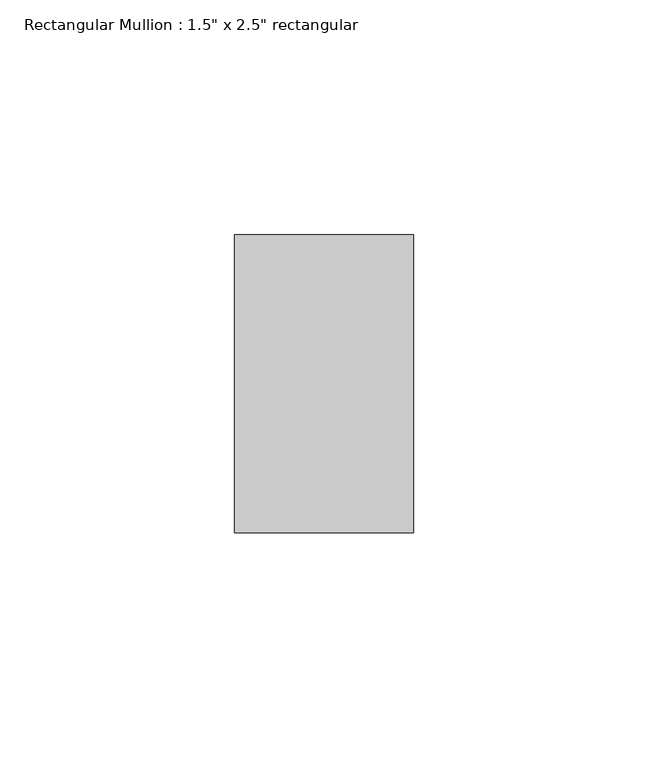
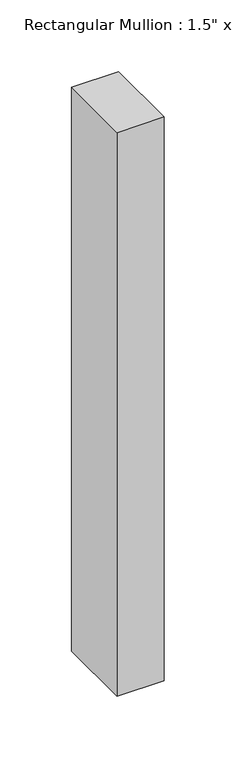
"""IFC4 building model written with IfcOpenShell, lengths in millimetres: member geometry."""

from ifc_helpers import new_model, si_unit, frame, origin, place, context, project, spatial, polyline, outline, extrude, source, transform, mapped, element, save


def member_6a2c51b8(model_context):
    return source(origin(), model_context, "Body", "SweptSolid", [
        extrude(outline(polyline([(19.05, 31.75), (19.05, -31.75), (-19.05, -31.75), (-19.05, 31.75), (19.05, 31.75)])), frame((0.0, 0.0, -480.1854569), z_axis=(0.0, 0.0, 1.0), x_axis=(1.0, 0.0, 0.0)), (0.0, 0.0, 1.0), 480.1854569),
    ])


if __name__ == "__main__":
    model = new_model("IFC4")
    model_context = context("Model", 3, world=origin())
    ifc_project = project(units=[si_unit("LENGTHUNIT", "METRE", prefix="MILLI")], contexts=[model_context])
    site = spatial("IfcSite", under=ifc_project)
    building = spatial("IfcBuilding", under=site)
    placement = place(None, origin())
    member_shape = member_6a2c51b8(model_context)
    element("IfcMember", 1, ObjectType="Rectangular Mullion : 1.5\" x 2.5\" rectangular", at=placement, inside=building, context=model_context, shape_type="MappedRepresentation", body=[
        mapped(member_shape, transform((0.0, 0.0, 0.0), x_axis=(1.0, 0.0, 0.0), y_axis=(0.0, 1.0, 0.0), z_axis=(0.0, 0.0, 1.0))),
    ])
    save(model, "model.ifc")

# Revit data of these elements
# Type "Rectangular Mullion : 1.5\" x 2.5\" rectangular"
#   built-in parameter 1007304 = 0.208333 (stored number, unit not read)
#   built-in parameter 1007301 = 0.0625 (stored number, unit not read)
#   built-in parameter 1007300 = 0.0625 (stored number, unit not read)
# Element 1 (IfcMember, "Rectangular Mullion : 1.5\" x 2.5\" rectangular")
#   Materials on its faces: "Leather - Black"
# Materials
#   "Leather - Black": class "Generic", colour RGB 40 40 40, transparency 0, Cost = 0
